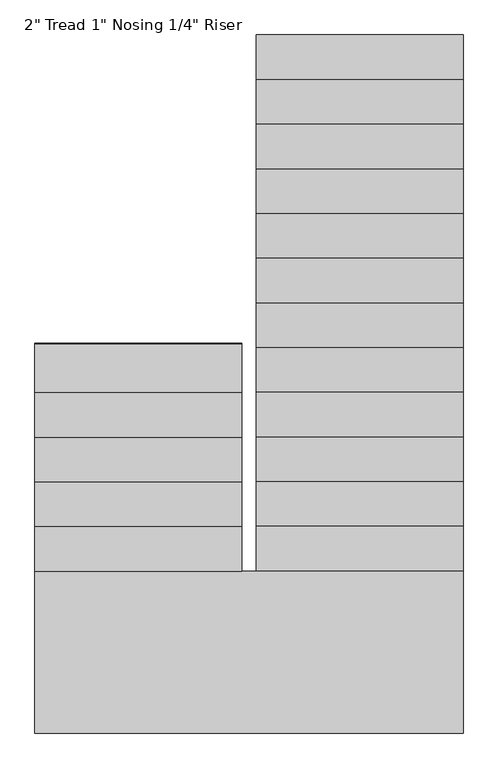
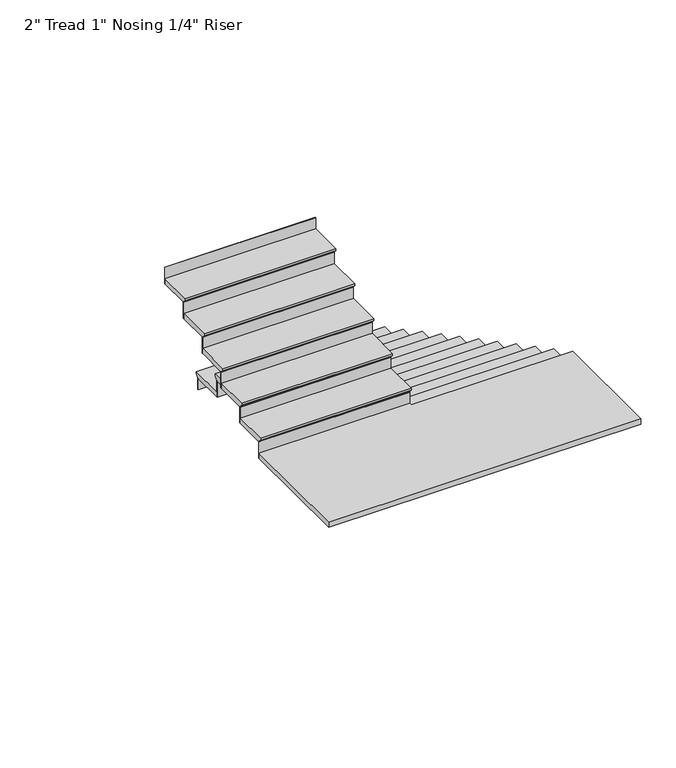
"""IFC4 building model written with IfcOpenShell, lengths in millimetres: stair flight geometry."""

from ifc_helpers import new_model, si_unit, origin, place, context, project, spatial, faceted_brep, source, transform, mapped, element, save


def stair_flight_69588459(model_context):
    return source(origin(), model_context, "Body", "Brep", [
        faceted_brep([(-1121.360394, -1150.2831508, 3189.3710526), (-1121.360394, -1150.2831508, 3208.4210526), (288.339606, -1150.2831508, 3208.4210526), (288.339606, -1150.2831508, 3189.3710526), (-1121.360394, -1175.6831508, 3163.9710526), (288.339606, -1175.6831508, 3163.9710526), (-1121.360394, -1480.4831508, 3208.4210526), (288.339606, -1480.4831508, 3208.4210526), (288.339606, -1175.6831508, 3157.6210526), (288.339606, -1480.4831508, 3157.6210526), (-1121.360394, -1480.4831508, 3157.6210526), (-1121.360394, -1175.6831508, 3157.6210526)], [[[0, 1, 2, 3]], [[4, 0, 3, 5]], [[2, 1, 6, 7]], [[8, 9, 10, 11]], [[2, 7, 9, 8, 5, 3]], [[8, 11, 4, 5]], [[6, 1, 0, 4, 11, 10]], [[7, 6, 10, 9]]]),
        faceted_brep([(-1121.360394, -1175.6831508, 3157.6210526), (-1121.360394, -1175.6831508, 3048.0), (-1121.360394, -1182.0331508, 3048.0), (-1121.360394, -1182.0331508, 3157.6210526), (288.339606, -1175.6831508, 3157.6210526), (288.339606, -1182.0331508, 3157.6210526), (288.339606, -1182.0331508, 3048.0), (288.339606, -1175.6831508, 3048.0)], [[[0, 1, 2, 3]], [[4, 5, 6, 7]], [[1, 0, 4, 7]], [[2, 1, 7, 6]], [[3, 2, 6, 5]], [[0, 3, 5, 4]]]),
        faceted_brep([(-1121.360394, -1480.4831508, 3318.0421053), (-1121.360394, -1480.4831508, 3157.6210526), (-1121.360394, -1486.8331508, 3157.6210526), (-1121.360394, -1486.8331508, 3318.0421053), (288.339606, -1480.4831508, 3318.0421053), (288.339606, -1486.8331508, 3318.0421053), (288.339606, -1486.8331508, 3157.6210526), (288.339606, -1480.4831508, 3157.6210526)], [[[0, 1, 2, 3]], [[4, 5, 6, 7]], [[1, 0, 4, 7]], [[2, 1, 7, 6]], [[3, 2, 6, 5]], [[0, 3, 5, 4]]]),
        faceted_brep([(288.339606, -1455.0831508, 3368.8421053), (-1121.360394, -1455.0831508, 3368.8421053), (-1121.360394, -1785.2831508, 3368.8421053), (288.339606, -1785.2831508, 3368.8421053), (288.339606, -1480.4831508, 3318.0421053), (288.339606, -1785.2831508, 3318.0421053), (-1121.360394, -1785.2831508, 3318.0421053), (-1121.360394, -1480.4831508, 3318.0421053), (288.339606, -1480.4831508, 3324.3921053), (288.339606, -1455.0831508, 3349.7921053), (-1121.360394, -1480.4831508, 3324.3921053), (-1121.360394, -1455.0831508, 3349.7921053)], [[[0, 1, 2, 3]], [[4, 5, 6, 7]], [[0, 3, 5, 4, 8, 9]], [[4, 7, 10, 8]], [[2, 1, 11, 10, 7, 6]], [[3, 2, 6, 5]], [[11, 1, 0, 9]], [[10, 11, 9, 8]]]),
        faceted_brep([(-1121.360394, -1785.2831508, 3478.4631579), (-1121.360394, -1785.2831508, 3318.0421053), (-1121.360394, -1791.6331508, 3318.0421053), (-1121.360394, -1791.6331508, 3478.4631579), (288.339606, -1785.2831508, 3478.4631579), (288.339606, -1791.6331508, 3478.4631579), (288.339606, -1791.6331508, 3318.0421053), (288.339606, -1785.2831508, 3318.0421053)], [[[0, 1, 2, 3]], [[4, 5, 6, 7]], [[1, 0, 4, 7]], [[2, 1, 7, 6]], [[3, 2, 6, 5]], [[0, 3, 5, 4]]]),
        faceted_brep([(288.339606, -1759.8831508, 3529.2631579), (-1121.360394, -1759.8831508, 3529.2631579), (-1121.360394, -2090.0831508, 3529.2631579), (288.339606, -2090.0831508, 3529.2631579), (288.339606, -1785.2831508, 3478.4631579), (288.339606, -2090.0831508, 3478.4631579), (-1121.360394, -2090.0831508, 3478.4631579), (-1121.360394, -1785.2831508, 3478.4631579), (288.339606, -1785.2831508, 3484.8131579), (288.339606, -1759.8831508, 3510.2131579), (-1121.360394, -1785.2831508, 3484.8131579), (-1121.360394, -1759.8831508, 3510.2131579)], [[[0, 1, 2, 3]], [[4, 5, 6, 7]], [[0, 3, 5, 4, 8, 9]], [[4, 7, 10, 8]], [[2, 1, 11, 10, 7, 6]], [[3, 2, 6, 5]], [[11, 1, 0, 9]], [[10, 11, 9, 8]]]),
        faceted_brep([(-1121.360394, -2090.0831508, 3638.8842105), (-1121.360394, -2090.0831508, 3478.4631579), (-1121.360394, -2096.4331508, 3478.4631579), (-1121.360394, -2096.4331508, 3638.8842105), (288.339606, -2090.0831508, 3638.8842105), (288.339606, -2096.4331508, 3638.8842105), (288.339606, -2096.4331508, 3478.4631579), (288.339606, -2090.0831508, 3478.4631579)], [[[0, 1, 2, 3]], [[4, 5, 6, 7]], [[1, 0, 4, 7]], [[2, 1, 7, 6]], [[3, 2, 6, 5]], [[0, 3, 5, 4]]]),
        faceted_brep([(288.339606, -2064.6831508, 3689.6842105), (-1121.360394, -2064.6831508, 3689.6842105), (-1121.360394, -2394.8831508, 3689.6842105), (288.339606, -2394.8831508, 3689.6842105), (288.339606, -2090.0831508, 3638.8842105), (288.339606, -2394.8831508, 3638.8842105), (-1121.360394, -2394.8831508, 3638.8842105), (-1121.360394, -2090.0831508, 3638.8842105), (288.339606, -2090.0831508, 3645.2342105), (288.339606, -2064.6831508, 3670.6342105), (-1121.360394, -2090.0831508, 3645.2342105), (-1121.360394, -2064.6831508, 3670.6342105)], [[[0, 1, 2, 3]], [[4, 5, 6, 7]], [[0, 3, 5, 4, 8, 9]], [[4, 7, 10, 8]], [[2, 1, 11, 10, 7, 6]], [[3, 2, 6, 5]], [[11, 1, 0, 9]], [[10, 11, 9, 8]]]),
        faceted_brep([(-1121.360394, -2394.8831508, 3799.3052632), (-1121.360394, -2394.8831508, 3638.8842105), (-1121.360394, -2401.2331508, 3638.8842105), (-1121.360394, -2401.2331508, 3799.3052632), (288.339606, -2394.8831508, 3799.3052632), (288.339606, -2401.2331508, 3799.3052632), (288.339606, -2401.2331508, 3638.8842105), (288.339606, -2394.8831508, 3638.8842105)], [[[0, 1, 2, 3]], [[4, 5, 6, 7]], [[1, 0, 4, 7]], [[2, 1, 7, 6]], [[3, 2, 6, 5]], [[0, 3, 5, 4]]]),
        faceted_brep([(288.339606, -2369.4831508, 3850.1052632), (-1121.360394, -2369.4831508, 3850.1052632), (-1121.360394, -2699.6831508, 3850.1052632), (288.339606, -2699.6831508, 3850.1052632), (288.339606, -2394.8831508, 3799.3052632), (288.339606, -2699.6831508, 3799.3052632), (-1121.360394, -2699.6831508, 3799.3052632), (-1121.360394, -2394.8831508, 3799.3052632), (288.339606, -2394.8831508, 3805.6552632), (288.339606, -2369.4831508, 3831.0552632), (-1121.360394, -2394.8831508, 3805.6552632), (-1121.360394, -2369.4831508, 3831.0552632)], [[[0, 1, 2, 3]], [[4, 5, 6, 7]], [[0, 3, 5, 4, 8, 9]], [[4, 7, 10, 8]], [[2, 1, 11, 10, 7, 6]], [[3, 2, 6, 5]], [[11, 1, 0, 9]], [[10, 11, 9, 8]]]),
        faceted_brep([(-1121.360394, -2699.6831508, 3959.7263158), (-1121.360394, -2699.6831508, 3799.3052632), (-1121.360394, -2706.0331508, 3799.3052632), (-1121.360394, -2706.0331508, 3959.7263158), (288.339606, -2699.6831508, 3959.7263158), (288.339606, -2706.0331508, 3959.7263158), (288.339606, -2706.0331508, 3799.3052632), (288.339606, -2699.6831508, 3799.3052632)], [[[0, 1, 2, 3]], [[4, 5, 6, 7]], [[1, 0, 4, 7]], [[2, 1, 7, 6]], [[3, 2, 6, 5]], [[0, 3, 5, 4]]]),
        faceted_brep([(288.339606, -2674.2831508, 4010.5263158), (-1121.360394, -2674.2831508, 4010.5263158), (-1121.360394, -3004.4831508, 4010.5263158), (288.339606, -3004.4831508, 4010.5263158), (288.339606, -2699.6831508, 3959.7263158), (288.339606, -3004.4831508, 3959.7263158), (-1121.360394, -3004.4831508, 3959.7263158), (-1121.360394, -2699.6831508, 3959.7263158), (288.339606, -2699.6831508, 3966.0763158), (288.339606, -2674.2831508, 3991.4763158), (-1121.360394, -2699.6831508, 3966.0763158), (-1121.360394, -2674.2831508, 3991.4763158)], [[[0, 1, 2, 3]], [[4, 5, 6, 7]], [[0, 3, 5, 4, 8, 9]], [[4, 7, 10, 8]], [[2, 1, 11, 10, 7, 6]], [[3, 2, 6, 5]], [[11, 1, 0, 9]], [[10, 11, 9, 8]]]),
        faceted_brep([(-1121.360394, -3004.4831508, 4120.1473684), (-1121.360394, -3004.4831508, 3959.7263158), (-1121.360394, -3010.8331508, 3959.7263158), (-1121.360394, -3010.8331508, 4120.1473684), (288.339606, -3004.4831508, 4120.1473684), (288.339606, -3010.8331508, 4120.1473684), (288.339606, -3010.8331508, 3959.7263158), (288.339606, -3004.4831508, 3959.7263158)], [[[0, 1, 2, 3]], [[4, 5, 6, 7]], [[1, 0, 4, 7]], [[2, 1, 7, 6]], [[3, 2, 6, 5]], [[0, 3, 5, 4]]]),
        faceted_brep([(288.339606, -2979.0831508, 4170.9473684), (-1121.360394, -2979.0831508, 4170.9473684), (-1121.360394, -3309.2831508, 4170.9473684), (288.339606, -3309.2831508, 4170.9473684), (288.339606, -3004.4831508, 4120.1473684), (288.339606, -3309.2831508, 4120.1473684), (-1121.360394, -3309.2831508, 4120.1473684), (-1121.360394, -3004.4831508, 4120.1473684), (288.339606, -3004.4831508, 4126.4973684), (288.339606, -2979.0831508, 4151.8973684), (-1121.360394, -3004.4831508, 4126.4973684), (-1121.360394, -2979.0831508, 4151.8973684)], [[[0, 1, 2, 3]], [[4, 5, 6, 7]], [[0, 3, 5, 4, 8, 9]], [[4, 7, 10, 8]], [[2, 1, 11, 10, 7, 6]], [[3, 2, 6, 5]], [[11, 1, 0, 9]], [[10, 11, 9, 8]]]),
        faceted_brep([(-1121.360394, -3309.2831508, 4280.5684211), (-1121.360394, -3309.2831508, 4120.1473684), (-1121.360394, -3315.6331508, 4120.1473684), (-1121.360394, -3315.6331508, 4280.5684211), (288.339606, -3309.2831508, 4280.5684211), (288.339606, -3315.6331508, 4280.5684211), (288.339606, -3315.6331508, 4120.1473684), (288.339606, -3309.2831508, 4120.1473684)], [[[0, 1, 2, 3]], [[4, 5, 6, 7]], [[1, 0, 4, 7]], [[2, 1, 7, 6]], [[3, 2, 6, 5]], [[0, 3, 5, 4]]]),
        faceted_brep([(288.339606, -3283.8831508, 4331.3684211), (-1121.360394, -3283.8831508, 4331.3684211), (-1121.360394, -3614.0831508, 4331.3684211), (288.339606, -3614.0831508, 4331.3684211), (288.339606, -3309.2831508, 4280.5684211), (288.339606, -3614.0831508, 4280.5684211), (-1121.360394, -3614.0831508, 4280.5684211), (-1121.360394, -3309.2831508, 4280.5684211), (288.339606, -3309.2831508, 4286.9184211), (288.339606, -3283.8831508, 4312.3184211), (-1121.360394, -3309.2831508, 4286.9184211), (-1121.360394, -3283.8831508, 4312.3184211)], [[[0, 1, 2, 3]], [[4, 5, 6, 7]], [[0, 3, 5, 4, 8, 9]], [[4, 7, 10, 8]], [[2, 1, 11, 10, 7, 6]], [[3, 2, 6, 5]], [[11, 1, 0, 9]], [[10, 11, 9, 8]]]),
        faceted_brep([(-1121.360394, -3614.0831508, 4440.9894737), (-1121.360394, -3614.0831508, 4280.5684211), (-1121.360394, -3620.4331508, 4280.5684211), (-1121.360394, -3620.4331508, 4440.9894737), (288.339606, -3614.0831508, 4440.9894737), (288.339606, -3620.4331508, 4440.9894737), (288.339606, -3620.4331508, 4280.5684211), (288.339606, -3614.0831508, 4280.5684211)], [[[0, 1, 2, 3]], [[4, 5, 6, 7]], [[1, 0, 4, 7]], [[2, 1, 7, 6]], [[3, 2, 6, 5]], [[0, 3, 5, 4]]]),
        faceted_brep([(288.339606, -3588.6831508, 4491.7894737), (-1121.360394, -3588.6831508, 4491.7894737), (-1121.360394, -3918.8831508, 4491.7894737), (288.339606, -3918.8831508, 4491.7894737), (288.339606, -3614.0831508, 4440.9894737), (288.339606, -3918.8831508, 4440.9894737), (-1121.360394, -3918.8831508, 4440.9894737), (-1121.360394, -3614.0831508, 4440.9894737), (288.339606, -3614.0831508, 4447.3394737), (288.339606, -3588.6831508, 4472.7394737), (-1121.360394, -3614.0831508, 4447.3394737), (-1121.360394, -3588.6831508, 4472.7394737)], [[[0, 1, 2, 3]], [[4, 5, 6, 7]], [[0, 3, 5, 4, 8, 9]], [[4, 7, 10, 8]], [[2, 1, 11, 10, 7, 6]], [[3, 2, 6, 5]], [[11, 1, 0, 9]], [[10, 11, 9, 8]]]),
        faceted_brep([(-1121.360394, -3918.8831508, 4601.4105263), (-1121.360394, -3918.8831508, 4440.9894737), (-1121.360394, -3925.2331508, 4440.9894737), (-1121.360394, -3925.2331508, 4601.4105263), (288.339606, -3918.8831508, 4601.4105263), (288.339606, -3925.2331508, 4601.4105263), (288.339606, -3925.2331508, 4440.9894737), (288.339606, -3918.8831508, 4440.9894737)], [[[0, 1, 2, 3]], [[4, 5, 6, 7]], [[1, 0, 4, 7]], [[2, 1, 7, 6]], [[3, 2, 6, 5]], [[0, 3, 5, 4]]]),
        faceted_brep([(288.339606, -3893.4831508, 4652.2105263), (-1121.360394, -3893.4831508, 4652.2105263), (-1121.360394, -4223.6831508, 4652.2105263), (288.339606, -4223.6831508, 4652.2105263), (288.339606, -3918.8831508, 4601.4105263), (288.339606, -4223.6831508, 4601.4105263), (-1121.360394, -4223.6831508, 4601.4105263), (-1121.360394, -3918.8831508, 4601.4105263), (288.339606, -3918.8831508, 4607.7605263), (288.339606, -3893.4831508, 4633.1605263), (-1121.360394, -3918.8831508, 4607.7605263), (-1121.360394, -3893.4831508, 4633.1605263)], [[[0, 1, 2, 3]], [[4, 5, 6, 7]], [[0, 3, 5, 4, 8, 9]], [[4, 7, 10, 8]], [[2, 1, 11, 10, 7, 6]], [[3, 2, 6, 5]], [[11, 1, 0, 9]], [[10, 11, 9, 8]]]),
        faceted_brep([(-1121.360394, -4223.6831508, 4761.8315789), (-1121.360394, -4223.6831508, 4601.4105263), (-1121.360394, -4230.0331508, 4601.4105263), (-1121.360394, -4230.0331508, 4761.8315789), (288.339606, -4223.6831508, 4761.8315789), (288.339606, -4230.0331508, 4761.8315789), (288.339606, -4230.0331508, 4601.4105263), (288.339606, -4223.6831508, 4601.4105263)], [[[0, 1, 2, 3]], [[4, 5, 6, 7]], [[1, 0, 4, 7]], [[2, 1, 7, 6]], [[3, 2, 6, 5]], [[0, 3, 5, 4]]]),
        faceted_brep([(288.339606, -4198.2831508, 4812.6315789), (-1121.360394, -4198.2831508, 4812.6315789), (-1121.360394, -4528.4831508, 4812.6315789), (288.339606, -4528.4831508, 4812.6315789), (288.339606, -4223.6831508, 4761.8315789), (288.339606, -4528.4831508, 4761.8315789), (-1121.360394, -4528.4831508, 4761.8315789), (-1121.360394, -4223.6831508, 4761.8315789), (288.339606, -4223.6831508, 4768.1815789), (288.339606, -4198.2831508, 4793.5815789), (-1121.360394, -4223.6831508, 4768.1815789), (-1121.360394, -4198.2831508, 4793.5815789)], [[[0, 1, 2, 3]], [[4, 5, 6, 7]], [[0, 3, 5, 4, 8, 9]], [[4, 7, 10, 8]], [[2, 1, 11, 10, 7, 6]], [[3, 2, 6, 5]], [[11, 1, 0, 9]], [[10, 11, 9, 8]]]),
        faceted_brep([(-1121.360394, -4528.4831508, 4922.2526316), (-1121.360394, -4528.4831508, 4761.8315789), (-1121.360394, -4534.8331508, 4761.8315789), (-1121.360394, -4534.8331508, 4922.2526316), (288.339606, -4528.4831508, 4922.2526316), (288.339606, -4534.8331508, 4922.2526316), (288.339606, -4534.8331508, 4761.8315789), (288.339606, -4528.4831508, 4761.8315789)], [[[0, 1, 2, 3]], [[4, 5, 6, 7]], [[1, 0, 4, 7]], [[2, 1, 7, 6]], [[3, 2, 6, 5]], [[0, 3, 5, 4]]]),
        faceted_brep([(288.339606, -4503.0831508, 4973.0526316), (-1121.360394, -4503.0831508, 4973.0526316), (-1121.360394, -4833.2831508, 4973.0526316), (288.339606, -4833.2831508, 4973.0526316), (288.339606, -4528.4831508, 4922.2526316), (288.339606, -4833.2831508, 4922.2526316), (-1121.360394, -4833.2831508, 4922.2526316), (-1121.360394, -4528.4831508, 4922.2526316), (288.339606, -4528.4831508, 4928.6026316), (288.339606, -4503.0831508, 4954.0026316), (-1121.360394, -4528.4831508, 4928.6026316), (-1121.360394, -4503.0831508, 4954.0026316)], [[[0, 1, 2, 3]], [[4, 5, 6, 7]], [[0, 3, 5, 4, 8, 9]], [[4, 7, 10, 8]], [[2, 1, 11, 10, 7, 6]], [[3, 2, 6, 5]], [[11, 1, 0, 9]], [[10, 11, 9, 8]]]),
        faceted_brep([(-1121.360394, -4833.2831508, 5082.6736842), (-1121.360394, -4833.2831508, 4922.2526316), (-1121.360394, -4839.6331508, 4922.2526316), (-1121.360394, -4839.6331508, 5082.6736842), (288.339606, -4833.2831508, 5082.6736842), (288.339606, -4839.6331508, 5082.6736842), (288.339606, -4839.6331508, 4922.2526316), (288.339606, -4833.2831508, 4922.2526316)], [[[0, 1, 2, 3]], [[4, 5, 6, 7]], [[1, 0, 4, 7]], [[2, 1, 7, 6]], [[3, 2, 6, 5]], [[0, 3, 5, 4]]]),
        faceted_brep([(-2632.660394, -4782.4831508, 5133.4736842), (-2632.660394, -5912.7831508, 5133.4736842), (288.339606, -5912.7831508, 5133.4736842), (288.339606, -4807.8831508, 5133.4736842), (-1222.960394, -4807.8831508, 5133.4736842), (-1222.960394, -4782.4831508, 5133.4736842), (-2632.660394, -5912.7831508, 5082.6736842), (-2632.660394, -4782.4831508, 5082.6736842), (-1222.960394, -4782.4831508, 5082.6736842), (-1222.960394, -4807.8831508, 5082.6736842), (-1121.360394, -4807.8831508, 5082.6736842), (-1121.360394, -4833.2831508, 5082.6736842), (288.339606, -4833.2831508, 5082.6736842), (288.339606, -5912.7831508, 5082.6736842), (288.339606, -4833.2831508, 5089.0236842), (288.339606, -4807.8831508, 5114.4236842), (-1121.360394, -4833.2831508, 5089.0236842), (-1121.360394, -4807.8831508, 5114.4236842)], [[[0, 1, 2, 3, 4, 5]], [[6, 7, 8, 9, 10, 11, 12, 13]], [[1, 0, 7, 6]], [[2, 1, 6, 13]], [[3, 2, 13, 12, 14, 15]], [[12, 11, 16, 14]], [[11, 10, 17, 16]], [[4, 3, 15, 17, 10, 9]], [[5, 4, 9, 8]], [[0, 5, 8, 7]], [[15, 14, 16, 17]]]),
        faceted_brep([(-1222.960394, -4782.4831508, 5243.0947368), (-1222.960394, -4782.4831508, 5082.6736842), (-1222.960394, -4776.1331508, 5082.6736842), (-1222.960394, -4776.1331508, 5243.0947368), (-2632.660394, -4782.4831508, 5243.0947368), (-2632.660394, -4776.1331508, 5243.0947368), (-2632.660394, -4776.1331508, 5082.6736842), (-2632.660394, -4782.4831508, 5082.6736842)], [[[0, 1, 2, 3]], [[4, 5, 6, 7]], [[1, 0, 4, 7]], [[2, 1, 7, 6]], [[3, 2, 6, 5]], [[0, 3, 5, 4]]]),
        faceted_brep([(-2632.660394, -4807.8831508, 5293.8947368), (-1222.960394, -4807.8831508, 5293.8947368), (-1222.960394, -4477.6831508, 5293.8947368), (-2632.660394, -4477.6831508, 5293.8947368), (-2632.660394, -4782.4831508, 5243.0947368), (-2632.660394, -4477.6831508, 5243.0947368), (-1222.960394, -4477.6831508, 5243.0947368), (-1222.960394, -4782.4831508, 5243.0947368), (-2632.660394, -4782.4831508, 5249.4447368), (-2632.660394, -4807.8831508, 5274.8447368), (-1222.960394, -4782.4831508, 5249.4447368), (-1222.960394, -4807.8831508, 5274.8447368)], [[[0, 1, 2, 3]], [[4, 5, 6, 7]], [[0, 3, 5, 4, 8, 9]], [[4, 7, 10, 8]], [[2, 1, 11, 10, 7, 6]], [[3, 2, 6, 5]], [[11, 1, 0, 9]], [[10, 11, 9, 8]]]),
        faceted_brep([(-1222.960394, -4477.6831508, 5403.5157895), (-1222.960394, -4477.6831508, 5243.0947368), (-1222.960394, -4471.3331508, 5243.0947368), (-1222.960394, -4471.3331508, 5403.5157895), (-2632.660394, -4477.6831508, 5403.5157895), (-2632.660394, -4471.3331508, 5403.5157895), (-2632.660394, -4471.3331508, 5243.0947368), (-2632.660394, -4477.6831508, 5243.0947368)], [[[0, 1, 2, 3]], [[4, 5, 6, 7]], [[1, 0, 4, 7]], [[2, 1, 7, 6]], [[3, 2, 6, 5]], [[0, 3, 5, 4]]]),
        faceted_brep([(-2632.660394, -4503.0831508, 5454.3157895), (-1222.960394, -4503.0831508, 5454.3157895), (-1222.960394, -4172.8831508, 5454.3157895), (-2632.660394, -4172.8831508, 5454.3157895), (-2632.660394, -4477.6831508, 5403.5157895), (-2632.660394, -4172.8831508, 5403.5157895), (-1222.960394, -4172.8831508, 5403.5157895), (-1222.960394, -4477.6831508, 5403.5157895), (-2632.660394, -4477.6831508, 5409.8657895), (-2632.660394, -4503.0831508, 5435.2657895), (-1222.960394, -4477.6831508, 5409.8657895), (-1222.960394, -4503.0831508, 5435.2657895)], [[[0, 1, 2, 3]], [[4, 5, 6, 7]], [[0, 3, 5, 4, 8, 9]], [[4, 7, 10, 8]], [[2, 1, 11, 10, 7, 6]], [[3, 2, 6, 5]], [[11, 1, 0, 9]], [[10, 11, 9, 8]]]),
        faceted_brep([(-1222.960394, -4172.8831508, 5563.9368421), (-1222.960394, -4172.8831508, 5403.5157895), (-1222.960394, -4166.5331508, 5403.5157895), (-1222.960394, -4166.5331508, 5563.9368421), (-2632.660394, -4172.8831508, 5563.9368421), (-2632.660394, -4166.5331508, 5563.9368421), (-2632.660394, -4166.5331508, 5403.5157895), (-2632.660394, -4172.8831508, 5403.5157895)], [[[0, 1, 2, 3]], [[4, 5, 6, 7]], [[1, 0, 4, 7]], [[2, 1, 7, 6]], [[3, 2, 6, 5]], [[0, 3, 5, 4]]]),
        faceted_brep([(-2632.660394, -4198.2831508, 5614.7368421), (-1222.960394, -4198.2831508, 5614.7368421), (-1222.960394, -3868.0831508, 5614.7368421), (-2632.660394, -3868.0831508, 5614.7368421), (-2632.660394, -4172.8831508, 5563.9368421), (-2632.660394, -3868.0831508, 5563.9368421), (-1222.960394, -3868.0831508, 5563.9368421), (-1222.960394, -4172.8831508, 5563.9368421), (-2632.660394, -4172.8831508, 5570.2868421), (-2632.660394, -4198.2831508, 5595.6868421), (-1222.960394, -4172.8831508, 5570.2868421), (-1222.960394, -4198.2831508, 5595.6868421)], [[[0, 1, 2, 3]], [[4, 5, 6, 7]], [[0, 3, 5, 4, 8, 9]], [[4, 7, 10, 8]], [[2, 1, 11, 10, 7, 6]], [[3, 2, 6, 5]], [[11, 1, 0, 9]], [[10, 11, 9, 8]]]),
        faceted_brep([(-1222.960394, -3868.0831508, 5724.3578947), (-1222.960394, -3868.0831508, 5563.9368421), (-1222.960394, -3861.7331508, 5563.9368421), (-1222.960394, -3861.7331508, 5724.3578947), (-2632.660394, -3868.0831508, 5724.3578947), (-2632.660394, -3861.7331508, 5724.3578947), (-2632.660394, -3861.7331508, 5563.9368421), (-2632.660394, -3868.0831508, 5563.9368421)], [[[0, 1, 2, 3]], [[4, 5, 6, 7]], [[1, 0, 4, 7]], [[2, 1, 7, 6]], [[3, 2, 6, 5]], [[0, 3, 5, 4]]]),
        faceted_brep([(-2632.660394, -3893.4831508, 5775.1578947), (-1222.960394, -3893.4831508, 5775.1578947), (-1222.960394, -3563.2831508, 5775.1578947), (-2632.660394, -3563.2831508, 5775.1578947), (-2632.660394, -3868.0831508, 5724.3578947), (-2632.660394, -3563.2831508, 5724.3578947), (-1222.960394, -3563.2831508, 5724.3578947), (-1222.960394, -3868.0831508, 5724.3578947), (-2632.660394, -3868.0831508, 5730.7078947), (-2632.660394, -3893.4831508, 5756.1078947), (-1222.960394, -3868.0831508, 5730.7078947), (-1222.960394, -3893.4831508, 5756.1078947)], [[[0, 1, 2, 3]], [[4, 5, 6, 7]], [[0, 3, 5, 4, 8, 9]], [[4, 7, 10, 8]], [[2, 1, 11, 10, 7, 6]], [[3, 2, 6, 5]], [[11, 1, 0, 9]], [[10, 11, 9, 8]]]),
        faceted_brep([(-1222.960394, -3563.2831508, 5884.7789474), (-1222.960394, -3563.2831508, 5724.3578947), (-1222.960394, -3556.9331508, 5724.3578947), (-1222.960394, -3556.9331508, 5884.7789474), (-2632.660394, -3563.2831508, 5884.7789474), (-2632.660394, -3556.9331508, 5884.7789474), (-2632.660394, -3556.9331508, 5724.3578947), (-2632.660394, -3563.2831508, 5724.3578947)], [[[0, 1, 2, 3]], [[4, 5, 6, 7]], [[1, 0, 4, 7]], [[2, 1, 7, 6]], [[3, 2, 6, 5]], [[0, 3, 5, 4]]]),
        faceted_brep([(-1222.960394, -3258.4831508, 6045.2), (-1222.960394, -3258.4831508, 5884.7789474), (-1222.960394, -3252.1331508, 5884.7789474), (-1222.960394, -3252.1331508, 6045.2), (-2632.660394, -3258.4831508, 6045.2), (-2632.660394, -3252.1331508, 6045.2), (-2632.660394, -3252.1331508, 5884.7789474), (-2632.660394, -3258.4831508, 5884.7789474)], [[[0, 1, 2, 3]], [[4, 5, 6, 7]], [[1, 0, 4, 7]], [[2, 1, 7, 6]], [[3, 2, 6, 5]], [[0, 3, 5, 4]]]),
        faceted_brep([(-2632.660394, -3588.6831508, 5935.5789474), (-1222.960394, -3588.6831508, 5935.5789474), (-1222.960394, -3258.4831508, 5935.5789474), (-2632.660394, -3258.4831508, 5935.5789474), (-2632.660394, -3563.2831508, 5884.7789474), (-2632.660394, -3258.4831508, 5884.7789474), (-1222.960394, -3258.4831508, 5884.7789474), (-1222.960394, -3563.2831508, 5884.7789474), (-2632.660394, -3563.2831508, 5891.1289474), (-2632.660394, -3588.6831508, 5916.5289474), (-1222.960394, -3563.2831508, 5891.1289474), (-1222.960394, -3588.6831508, 5916.5289474)], [[[0, 1, 2, 3]], [[4, 5, 6, 7]], [[0, 3, 5, 4, 8, 9]], [[4, 7, 10, 8]], [[2, 1, 11, 10, 7, 6]], [[3, 2, 6, 5]], [[11, 1, 0, 9]], [[10, 11, 9, 8]]]),
    ])


if __name__ == "__main__":
    model = new_model("IFC4")
    model_context = context("Model", 3, world=origin())
    ifc_project = project(units=[si_unit("LENGTHUNIT", "METRE", prefix="MILLI")], contexts=[model_context])
    site = spatial("IfcSite", under=ifc_project)
    building = spatial("IfcBuilding", under=site)
    placement = place(None, origin())
    stair_flight_shape = stair_flight_69588459(model_context)
    element("IfcStairFlight", 1, ObjectType="2\" Tread 1\" Nosing 1/4\" Riser", at=placement, inside=building, context=model_context, shape_type="MappedRepresentation", body=[
        mapped(stair_flight_shape, transform((0.0, 0.0, 0.0), x_axis=(1.0, 0.0, 0.0), y_axis=(0.0, 1.0, 0.0), z_axis=(0.0, 0.0, 1.0))),
    ])
    save(model, "model.ifc")
